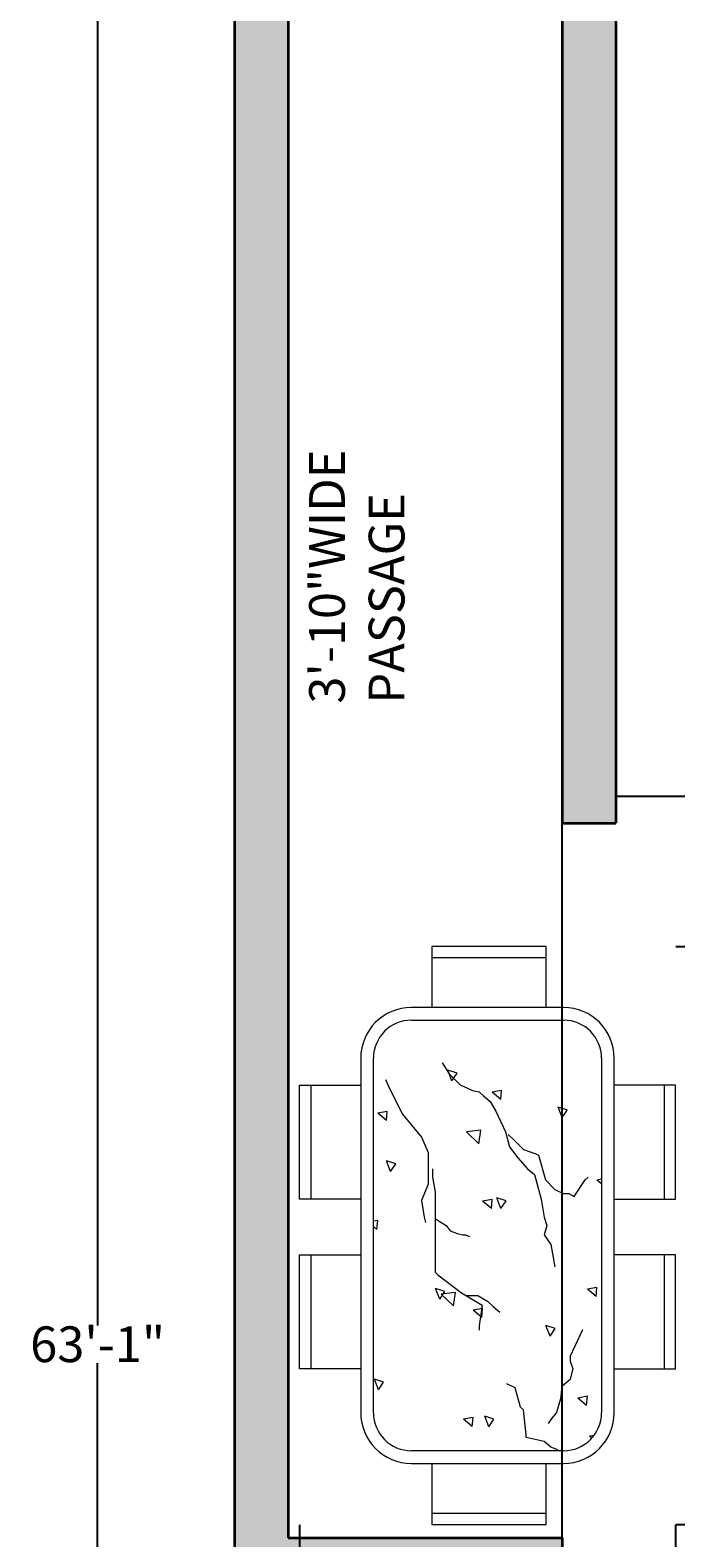
# Model space of a CAD drawing. Units: inches. Extents: x -16 to 587, y -783 to 64.
# Tile 10 of 14: x -16 to 92, y -392 to -138. Entities that reach past the tile are written whole.
import ezdxf

# ---------------------------------------------------------------- set-up
doc = ezdxf.new("R2010")
doc.units = ezdxf.units.IN
doc.header["$MEASUREMENT"] = 0
for name, color, linetype, lineweight in [('A-ANNO-DIMS', 2, 'Continuous', 18), ('A-AREA-IDEN', 7, 'Continuous', 18), ('A-DOOR', 3, 'Continuous', 25), ('A-FURN', 8, 'Continuous', 18), ('A-WALL', 7, 'Continuous', 35), ('A-WALL-PATT', 23, 'Continuous', 13)]:
    doc.layers.add(name, color=color, linetype=linetype, lineweight=lineweight)
doc.styles.get("Standard").update_dxf_attribs({"font": 'arial.ttf'})
doc.dimstyles.get("Standard").update_dxf_attribs({"dimtxt": 0.18, "dimasz": 0.18, "dimexe": 0.18, "dimexo": 0.0625, "dimgap": 0.09, "dimtad": 0, "dimtih": 1, "dimtoh": 1, "dimdec": 0, "dimzin": 0, "dimdsep": 46, "dimlunit": 3, "dimtxsty": 'Standard', "dimcen": 0.09, "dimadec": 0, "dimazin": 0, "dimtfac": 1, "dimtdec": 0, "dimtofl": 0, "dimtmove": 0, "dimatfit": 3, "dimfxl": 1, "dimtolj": 1, "dimtzin": 0, "dimarcsym": 0})

# ---------------------------------------------------------------- blocks, each defined once
blk = doc.blocks.new('*D6')
at = {"layer": 'A-ANNO-DIMS', "color": 0, "lineweight": -2, "transparency": 16777216}
for p, q in [((18.02, 19.45), (-5.05, 19.45)), ((-4.87, 19.27), (-4.87, -355.9)), ((-4.87, -737.37), (-4.87, -362.21)), ((18.02, -737.55), (-5.05, -737.55))]:
    blk.add_line(p, q, dxfattribs=at)
at = {"layer": 'A-ANNO-DIMS', "color": 0, "transparency": 16777216}
for points in [[(-4.9, 19.27), (-4.84, 19.27), (-4.87, 19.45)], [(-4.9, -737.37), (-4.84, -737.37), (-4.87, -737.55)]]:
    blk.add_solid(points, dxfattribs=at)
at = {"layer": 'Defpoints', "color": 0, "transparency": 16777216}
for p in [(18.08, 19.45), (-4.87, -737.55), (18.08, -737.55)]:
    blk.add_point(p, dxfattribs=at)
at = {"layer": 'A-ANNO-DIMS', "color": 0, "transparency": 16777216, "insert": (-4.87, -359.05), "char_height": 6, "attachment_point": 5}
blk.add_mtext('\\A1;63\'-1"', dxfattribs=at)
blk = doc.blocks.new('DINING-TABLE-SIX')
for p, q in [((41.34, 97.05), (22.2, 97.05)), ((22.2, 97.05), (22.2, 86.8)), ((41.34, 86.8), (41.34, 97.05)), ((22.2, 95.18), (41.34, 95.18)), ((44.27, 86.8), (18.76, 86.8)), ((18.76, 84.68), (44.27, 84.68)), ((10.25, 78.3), (10.25, 18.76)), ((12.38, 18.76), (12.38, 78.3)), ((23.9, 77.51), (25.06, 75.66)), ((25.54, 74.52), (24.86, 76.31)), ((26.4, 75.79), (24.86, 76.31)), ((50.65, 78.3), (50.65, 18.76)), ((52.78, 18.76), (52.78, 78.3)), ((0, 54.61), (0, 73.75)), ((0, 73.75), (10.25, 73.75)), ((1.87, 73.75), (1.87, 54.61)), ((14.43, 74.74), (14.9, 73.58)), ((14.9, 73.58), (17.21, 68.96)), ((25.06, 75.66), (26.91, 73.81)), ((25.54, 74.52), (26.4, 75.79)), ((26.91, 73.81), (28.99, 72.89)), ((63.03, 73.75), (52.78, 73.75)), ((61.16, 73.75), (61.16, 54.61)), ((63.03, 54.61), (63.03, 73.75)), ((28.99, 72.89), (30.14, 72.66)), ((30.14, 72.66), (30.83, 71.96)), ((30.83, 71.96), (31.99, 71.04)), ((31.99, 71.04), (32.91, 69.42)), ((33.89, 72.89), (32.29, 72.59)), ((33.76, 71.36), (32.29, 72.59)), ((33.76, 71.36), (33.89, 72.89)), ((14.7, 69.35), (13.1, 69.05)), ((14.56, 67.82), (13.1, 69.05)), ((14.56, 67.82), (14.7, 69.35)), ((17.21, 68.96), (20.44, 65.03)), ((32.91, 69.42), (34.53, 65.95)), ((44.91, 69.58), (43.36, 70.1)), ((44.05, 68.31), (43.36, 70.1)), ((44.05, 68.31), (44.9, 69.58)), ((30.4, 66.21), (27.97, 65.93)), ((30.04, 63.94), (27.97, 65.93)), ((30.04, 63.94), (30.4, 66.21)), ((34.53, 65.95), (35.22, 63.41)), ((20.44, 65.03), (21.59, 62.48)), ((34.99, 65.49), (35.91, 64.56)), ((35.22, 63.41), (36.61, 61.56)), ((35.91, 64.56), (37.53, 62.94)), ((15.27, 59.29), (14.58, 61.08)), ((16.13, 60.56), (14.59, 61.08)), ((21.59, 62.48), (21.59, 57.16)), ((36.61, 61.56), (38.22, 59.71)), ((37.53, 62.94), (39.61, 62.25)), ((39.61, 62.25), (40.07, 62.02)), ((40.07, 62.02), (41.23, 57.86)), ((15.27, 59.29), (16.13, 60.56)), ((22.29, 59.71), (22.29, 58.32)), ((22.29, 58.32), (22.75, 55.78)), ((38.22, 59.71), (39.38, 58.78)), ((39.38, 58.78), (40.53, 54.62)), ((47.92, 57.86), (48.39, 58.32)), ((21.59, 57.16), (20.44, 54.39)), ((22.75, 55.78), (22.75, 42.37)), ((41.23, 57.86), (42.84, 56.24)), ((42.84, 56.24), (44.23, 55.55)), ((46.08, 55.08), (47.92, 57.86)), ((50.65, 57.18), (49.88, 57.83)), ((50.65, 57.97), (49.89, 57.83)), ((10.25, 54.61), (0, 54.61)), ((20.44, 54.39), (20.9, 51.61)), ((32.29, 54.58), (30.69, 54.29)), ((32.16, 53.06), (30.69, 54.29)), ((32.16, 53.06), (32.29, 54.58)), ((33.77, 53.08), (33.09, 54.87)), ((34.63, 54.35), (33.09, 54.87)), ((33.77, 53.08), (34.63, 54.35)), ((40.53, 54.62), (41, 51.61)), ((44.23, 55.55), (45.15, 55.55)), ((45.15, 55.55), (46.08, 55.08)), ((52.78, 54.61), (63.03, 54.61)), ((13.1, 51.04), (12.38, 50.91)), ((12.96, 49.52), (13.1, 51.04)), ((20.9, 51.61), (21.13, 50.69)), ((22.74, 51.39), (23.43, 50.92)), ((23.43, 50.92), (24.59, 50.23)), ((41, 51.61), (41.46, 50.23)), ((12.96, 49.52), (12.38, 50.01)), ((24.59, 50.23), (25.28, 49.31)), ((25.28, 49.31), (26.44, 48.84)), ((26.44, 48.84), (27.36, 48.61)), ((27.36, 48.61), (27.82, 48.61)), ((27.82, 48.61), (28.51, 48.38)), ((41.46, 50.23), (41, 48.61)), ((41, 48.61), (42.15, 46.99)), ((42.15, 46.99), (42.84, 43.29)), ((0, 26.11), (0, 45.25)), ((0, 45.25), (10.25, 45.25)), ((1.87, 45.25), (1.87, 26.11)), ((63.03, 45.25), (52.78, 45.25)), ((61.16, 45.25), (61.16, 26.11)), ((63.03, 26.11), (63.03, 45.25)), ((22.75, 42.37), (23.21, 41.9)), ((23.21, 41.9), (27.14, 38.9)), ((23.5, 37.85), (22.81, 39.64)), ((24.36, 39.12), (22.82, 39.64)), ((23.5, 37.85), (24.36, 39.12)), ((26.17, 38.97), (23.75, 38.69)), ((25.82, 36.7), (23.75, 38.69)), ((25.82, 36.7), (26.17, 38.97)), ((27.14, 38.9), (30.6, 36.82)), ((27.83, 38.43), (29.91, 38.43)), ((29.91, 38.43), (31.53, 37.51)), ((49.88, 39.82), (48.28, 39.53)), ((49.75, 38.3), (48.28, 39.53)), ((49.75, 38.3), (49.88, 39.82)), ((30.69, 36.28), (29.09, 35.99)), ((30.56, 34.75), (29.09, 35.98)), ((30.6, 36.82), (30.14, 33.35)), ((30.56, 34.75), (30.69, 36.28)), ((31.53, 37.51), (32.45, 36.58)), ((32.45, 36.58), (33.6, 35.66)), ((30.14, 33.35), (30.14, 32.65)), ((42.01, 31.64), (41.32, 33.43)), ((42.86, 32.91), (41.32, 33.43)), ((42.01, 31.64), (42.86, 32.91)), ((47.45, 32.66), (45.37, 28.26)), ((45.37, 28.26), (45.37, 27.34)), ((10.25, 26.11), (0, 26.11)), ((45.37, 27.34), (45.84, 26.18)), ((45.84, 26.18), (45.37, 24.33)), ((52.78, 26.11), (63.03, 26.11)), ((13.23, 22.62), (12.54, 24.41)), ((14.08, 23.89), (12.54, 24.41)), ((13.23, 22.62), (14.08, 23.89)), ((36.14, 22.94), (34.76, 23.64)), ((37.07, 19.7), (36.14, 22.94)), ((43.99, 23.18), (43.76, 21.1)), ((45.37, 24.33), (43.99, 23.18)), ((43.76, 21.1), (43.07, 18.78)), ((48.28, 21.52), (46.68, 21.22)), ((48.15, 19.99), (46.68, 21.22)), ((48.15, 19.99), (48.28, 21.52)), ((29.09, 17.98), (27.49, 17.68)), ((28.95, 16.45), (29.09, 17.98)), ((31.73, 16.41), (31.05, 18.2)), ((32.59, 17.68), (31.05, 18.2)), ((37.53, 19.24), (37.07, 19.7)), ((37.99, 15.08), (37.53, 19.24)), ((43.07, 18.78), (42.14, 17.63)), ((28.95, 16.45), (27.49, 17.68)), ((31.73, 16.41), (32.59, 17.68)), ((42.14, 17.63), (41.68, 16.93)), ((37.99, 14.62), (37.99, 15.08)), ((41, 13.92), (37.99, 14.62)), ((42.15, 13), (41, 13.92)), ((43.3, 12.54), (42.15, 13)), ((49.38, 14.93), (48.61, 14.84)), ((49, 14.47), (48.61, 14.84)), ((44.27, 12.38), (18.76, 12.38)), ((18.76, 10.25), (44.27, 10.25)), ((22.2, 10.25), (22.2, 0)), ((41.34, 0), (41.34, 10.25)), ((41.34, 1.87), (22.2, 1.87)), ((22.2, 0), (41.34, 0))]:
    blk.add_line(p, q)
for centre, radius, start, end in [((18.76, 78.3), 8.51, 90, 180), ((44.27, 78.3), 8.51, 0, 90), ((18.76, 78.3), 6.38, 90, 180), ((44.27, 78.3), 6.38, 0, 90), ((18.76, 18.76), 8.51, 180, 270), ((18.76, 18.76), 6.38, 180, 270), ((44.27, 18.76), 6.38, 270, 0), ((44.27, 18.76), 8.51, 270, 0)]:
    blk.add_arc(centre, radius, start, end)
blk = doc.blocks.new('*D36')
at = {"layer": 'A-ANNO-DIMS', "color": 0, "lineweight": -2, "transparency": 16777216}
for p, q in [((92.12, -292.26), (106.79, -292.26)), ((106.61, -292.44), (106.61, -340.6)), ((106.61, -389.13), (106.61, -340.97)), ((92.12, -389.31), (106.79, -389.31))]:
    blk.add_line(p, q, dxfattribs=at)
at = {"layer": 'A-ANNO-DIMS', "color": 0, "transparency": 16777216}
for points in [[(106.58, -292.44), (106.64, -292.44), (106.61, -292.26)], [(106.58, -389.13), (106.64, -389.13), (106.61, -389.31)]]:
    blk.add_solid(points, dxfattribs=at)
at = {"layer": 'Defpoints', "color": 0, "transparency": 16777216}
for p in [(92.05, -292.26), (106.61, -292.26), (92.05, -389.31)]:
    blk.add_point(p, dxfattribs=at)
at = {"layer": 'A-ANNO-DIMS', "color": 0, "transparency": 16777216, "insert": (106.61, -340.78), "char_height": 0.18, "attachment_point": 5}
blk.add_mtext('\\A1;DINING SET 8\'-1" TYP.', dxfattribs=at)
blk = doc.blocks.new('*D37')
at = {"layer": 'A-ANNO-DIMS', "color": 0, "lineweight": -2, "transparency": 16777216}
for p, q in [((29.02, -389.37), (29.02, -404.05)), ((92.05, -389.37), (92.05, -404.05)), ((29.2, -403.87), (59.9, -403.87)), ((91.87, -403.87), (61.18, -403.87))]:
    blk.add_line(p, q, dxfattribs=at)
at = {"layer": 'A-ANNO-DIMS', "color": 0, "transparency": 16777216}
for points in [[(29.2, -403.84), (29.2, -403.9), (29.02, -403.87)], [(91.87, -403.84), (91.87, -403.9), (92.05, -403.87)]]:
    blk.add_solid(points, dxfattribs=at)
at = {"layer": 'Defpoints', "color": 0, "transparency": 16777216}
for p in [(29.02, -389.31), (92.05, -389.31), (92.05, -403.87)]:
    blk.add_point(p, dxfattribs=at)
at = {"layer": 'A-ANNO-DIMS', "color": 0, "transparency": 16777216, "insert": (60.54, -403.87), "char_height": 0.18, "attachment_point": 5}
blk.add_mtext('\\A1;5\'-3" TYP.', dxfattribs=at)
blk = doc.blocks.new('*D58')
at = {"layer": 'A-ANNO-DIMS', "color": 0, "lineweight": -2, "transparency": 16777216}
for p, q in [((73.08, -663.49), (73.08, 63.78)), ((73.26, 63.6), (90.75, 63.6)), ((108.9, 63.6), (91.41, 63.6)), ((109.08, -667.99), (109.08, 63.78))]:
    blk.add_line(p, q, dxfattribs=at)
at = {"layer": 'A-ANNO-DIMS', "color": 0, "transparency": 16777216}
for points in [[(73.26, 63.63), (73.26, 63.57), (73.08, 63.6)], [(108.9, 63.63), (108.9, 63.57), (109.08, 63.6)]]:
    blk.add_solid(points, dxfattribs=at)
at = {"layer": 'Defpoints', "color": 0, "transparency": 16777216}
for p in [(109.08, 63.6), (73.08, -663.55), (109.08, -668.05)]:
    blk.add_point(p, dxfattribs=at)
at = {"layer": 'A-ANNO-DIMS', "color": 0, "transparency": 16777216, "insert": (91.08, 63.6), "char_height": 0.18, "attachment_point": 5}
blk.add_mtext('\\A1;3\'-0"', dxfattribs=at)

msp = doc.modelspace()

# ---------------------------------------------------------------- hatches: boundary and pattern name
at = {"layer": 'A-WALL-PATT'}
h = msp.add_hatch(color=256, dxfattribs=at)
h.dxf.hatch_style = 1
h.paths.add_polyline_path([(137.08, -543.55), (137.08, -534.55), (118.08, -534.55), (118.08, -528.55), (109.08, -528.55), (109.08, -534.55), (109.08, -672.55), (118.08, -672.55), (118.08, -543.55)], flags=17)
h.paths.add_polyline_path([(27.08, -663.55), (27.08, -400.55), (73.08, -400.55), (73.08, -391.55), (27.08, -391.55), (27.08, 10.45), (48.75, 10.45), (171.08, 10.45), (171.08, -17.55), (180.08, -17.55), (180.08, 10.45), (228.08, 10.45), (228.08, -262.55), (206.41, -262.55), (118.08, -262.55), (118.08, -271.55), (228.08, -271.55), (228.08, -391.55), (154.08, -391.55), (154.08, -400.55), (228.08, -400.55), (228.08, -534.55), (209.08, -534.55), (209.08, -543.55), (237.08, -543.55), (237.08, 19.45), (18.08, 19.45), (18.08, -672.55), (73.08, -672.55), (73.08, -663.55)])
h.paths.add_polyline_path([(109.08, -486.55), (87.08, -486.55), (87.08, -495.55), (118.08, -495.55), (118.08, -400.55), (118.08, -391.55), (109.08, -391.55), (109.08, -400.55)], flags=17)
h = msp.add_hatch(color=256, dxfattribs=at)
h.dxf.hatch_style = 1
h.paths.add_polyline_path([(180.08, -41.55), (171.08, -41.55), (171.08, -78.55), (180.08, -78.55), (204.08, -78.55), (204.08, -69.55), (180.08, -69.55)], flags=17)
h.paths.add_polyline_path([(180.08, -130.55), (180.08, -121.55), (171.08, -121.55), (73.08, -121.55), (67.08, -121.55), (67.08, -130.55), (73.08, -130.55), (73.08, -271.55), (82.08, -271.55), (82.08, -130.55)], flags=17)
h.paths.add_polyline_path([(198.08, -307.55), (159.08, -307.55), (159.08, -355.55), (168.08, -355.55), (168.08, -316.55), (198.08, -316.55)], flags=17)

# ---------------------------------------------------------------- linework, layer by layer
at = {"layer": 'A-DOOR'}
msp.add_line((118.08, -267.05), (82.08, -267.05), dxfattribs=at)
at = {"layer": 'A-WALL'}
for p, q in [((18.08, 19.45), (18.08, -737.55)), ((27.08, 10.45), (27.08, -391.55)), ((73.08, -130.55), (73.08, -271.55)), ((82.08, -130.55), (82.08, -271.55)), ((73.08, -271.55), (82.08, -271.55)), ((27.08, -391.55), (73.08, -391.55)), ((73.08, -391.55), (73.08, -400.55))]:
    msp.add_line(p, q, dxfattribs=at)

# ---------------------------------------------------------------- block references
at = {"layer": 'A-FURN'}
msp.add_blockref('DINING-TABLE-SIX', (29.02, -389.31), dxfattribs=at)

# ---------------------------------------------------------------- texts
at = {"layer": 'A-AREA-IDEN', "insert": (30.61, -251.48), "char_height": 6, "attachment_point": 1, "rotation": 90}
msp.add_mtext('3\'-10"WIDE\\PPASSAGE', dxfattribs=at)

# ---------------------------------------------------------------- dimensions: what is measured, and where the dimension line sits
at = {"layer": 'A-ANNO-DIMS'}
dim = msp.add_linear_dim(base=(109.08, 63.6), p1=(73.08, -663.55), p2=(109.08, -668.05), dimstyle='Standard', override={"dimdec": 1, "dimlfac": 1, "dimrnd": 0, "dimzin": 1, "dimdsep": 46, "dimlunit": 4, "dimfrac": 2}, dxfattribs=at)
dim.commit()
dim.dimension.update_dxf_attribs({"geometry": '*D58', "text_midpoint": (91.08, 63.6)})
dim = msp.add_linear_dim(base=(-4.87, -737.55), p1=(18.08, 19.45), p2=(18.08, -737.55), angle=90, dimstyle='Standard', override={"dimtxt": 6, "dimclrd": 0, "dimclre": 0, "dimclrt": 0}, dxfattribs=at)
dim.commit()
dim.dimension.update_dxf_attribs({"geometry": '*D6', "text_midpoint": (-4.87, -359.05)})
dim = msp.add_linear_dim(base=(106.6123, -292.2563), p1=(92.0542, -389.3103), p2=(92.0542, -292.2563), angle=90, text='DINING SET <> TYP.', dimstyle='Standard', override={"dimdec": 1, "dimlfac": 1, "dimrnd": 0, "dimzin": 1, "dimdsep": 46, "dimlunit": 4, "dimfrac": 2}, dxfattribs=at)
dim.commit()
dim.dimension.update_dxf_attribs({"geometry": '*D36', "text_midpoint": (106.6123, -340.7833)})
dim = msp.add_linear_dim(base=(92.05, -403.87), p1=(29.02, -389.31), p2=(92.05, -389.31), text='<> TYP.', dimstyle='Standard', override={"dimdec": 1, "dimlfac": 1, "dimrnd": 0, "dimzin": 1, "dimdsep": 46, "dimlunit": 4, "dimfrac": 2}, dxfattribs=at)
dim.commit()
dim.dimension.update_dxf_attribs({"geometry": '*D37', "text_midpoint": (60.54, -403.87)})

doc.saveas('drawing.dxf')
